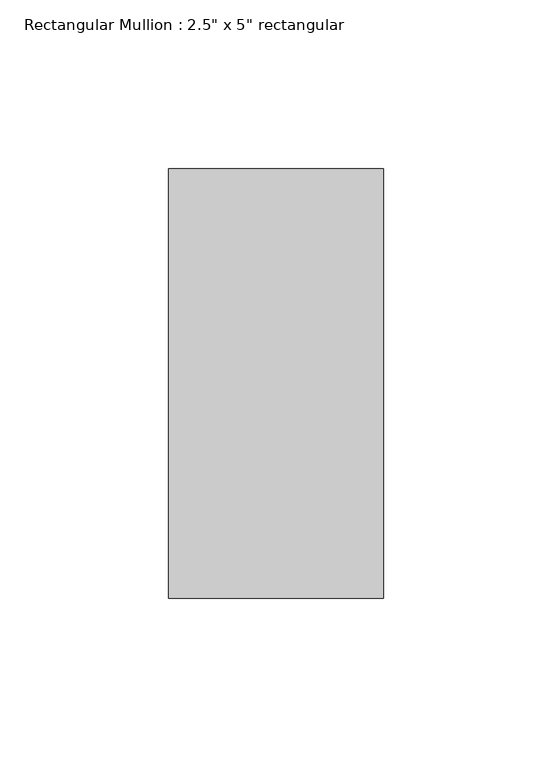
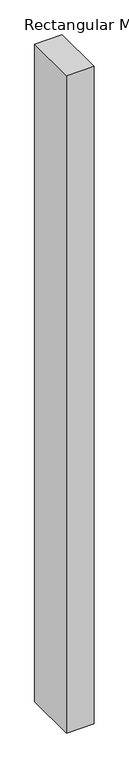
"""IFC4 building model written with IfcOpenShell, lengths in millimetres: member geometry."""

from ifc_helpers import new_model, si_unit, frame, origin, place, context, project, spatial, polyline, outline, extrude, source, transform, mapped, element, save


def member_46a214c3(model_context):
    return source(origin(), model_context, "Body", "SweptSolid", [
        extrude(outline(polyline([(0.0, 63.5), (0.0, -63.5), (-63.5, -63.5), (-63.5, 63.5), (0.0, 63.5)])), frame((0.0, 0.0, -1607.0454815), z_axis=(0.0, 0.0, 1.0), x_axis=(1.0, 0.0, 0.0)), (0.0, 0.0, 1.0), 1607.0454815),
    ])


if __name__ == "__main__":
    model = new_model("IFC4")
    model_context = context("Model", 3, world=origin())
    ifc_project = project(units=[si_unit("LENGTHUNIT", "METRE", prefix="MILLI")], contexts=[model_context])
    site = spatial("IfcSite", under=ifc_project)
    building = spatial("IfcBuilding", under=site)
    placement = place(None, origin())
    member_shape = member_46a214c3(model_context)
    element("IfcMember", 1, ObjectType="Rectangular Mullion : 2.5\" x 5\" rectangular", at=placement, inside=building, context=model_context, shape_type="MappedRepresentation", body=[
        mapped(member_shape, transform((0.0, 0.0, 0.0), x_axis=(1.0, 0.0, 0.0), y_axis=(0.0, 1.0, 0.0), z_axis=(0.0, 0.0, 1.0))),
    ])
    save(model, "model.ifc")

# Revit data of these elements
# Type "Rectangular Mullion : 2.5\" x 5\" rectangular"
#   built-in parameter 1007304 = 0.416667 (stored number, unit not read)
#   built-in parameter 1007301 = 0.104167 (stored number, unit not read)
#   built-in parameter 1007300 = 0.104167 (stored number, unit not read)
# Element 1 (IfcMember, "Rectangular Mullion : 2.5\" x 5\" rectangular")
#   Materials on its faces: "Aluminum"
# Materials
#   "Aluminum": class "Metal", colour RGB 247 247 247, transparency 0, Description = "Aluminum 6061", Cost = 0
